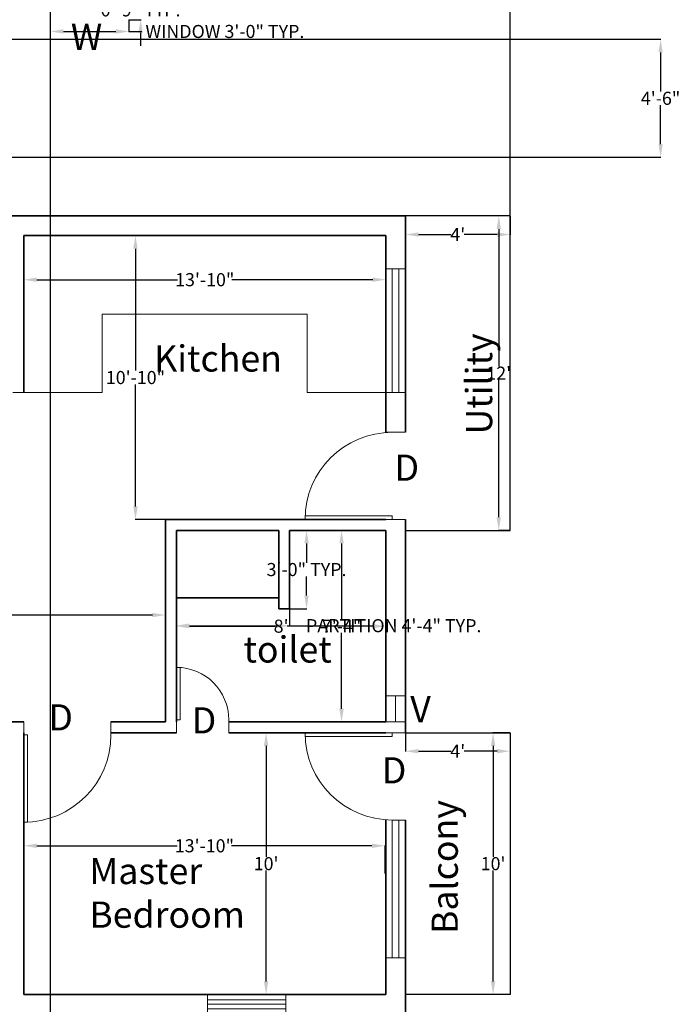
# Model space of a CAD drawing. Units: inches. Extents: x 1936 to 2761, y 1431 to 2889.
# Tile 4 of 6: x 2444 to 2747, y 1999 to 2451. Entities that reach past the tile are written whole.
import ezdxf

# ---------------------------------------------------------------- set-up
doc = ezdxf.new("R2010")
doc.units = ezdxf.units.IN
doc.header["$MEASUREMENT"] = 0
for name, color, linetype, lineweight in [('A-ANNO-DIMS', 172, 'Continuous', 13), ('A-ANNO-TEXT', 50, 'Continuous', 18), ('A-AREA-IDEN', 50, 'Continuous', 18), ('A-FLOR-EDGE', 4, 'Continuous', 25), ('A-FLOR-FIXT', 8, 'Continuous', 18), ('A-GLAZ', 3, 'Continuous', 18), ('A-WALL', 4, 'Continuous', 35), ('doors', 10, 'Continuous', 18)]:
    doc.layers.add(name, color=color, linetype=linetype, lineweight=lineweight)
doc.styles.get("Standard").update_dxf_attribs({"font": 'arial.ttf'})
doc.dimstyles.get("Standard").update_dxf_attribs({"dimtxt": 6, "dimasz": 6, "dimexe": 0.18, "dimexo": 0.0625, "dimgap": 0.09, "dimtad": 0, "dimtih": 1, "dimtoh": 1, "dimdec": 0, "dimzin": 0, "dimdsep": 46, "dimlunit": 3, "dimtxsty": 'Standard', "dimcen": 0.09, "dimadec": 0, "dimazin": 0, "dimtfac": 1, "dimtdec": 0, "dimtofl": 0, "dimtmove": 0, "dimatfit": 3, "dimfxl": 1, "dimtolj": 1, "dimtzin": 0, "dimarcsym": 0})

# ---------------------------------------------------------------- blocks, each defined once
blk = doc.blocks.new('*U2')
for p, q in [((0, 0), (0, 6)), ((40, 0), (40, 6))]:
    blk.add_line(p, q)
blk.add_lwpolyline([(0, 0), (0, -40), (1.75, -40), (1.75, 0)], close=True)
blk.add_arc((0, 0), 40, 270, 360)
blk = doc.blocks.new('*U3')
for p, q in [((0, 0), (0, -6)), ((24, 0), (24, -6))]:
    blk.add_line(p, q)
blk.add_lwpolyline([(0, 0), (0, 24), (1.75, 24), (1.75, 0)], close=True)
blk.add_arc((0, 0), 24, 0, 90)
blk = doc.blocks.new('*U5')
for p, q in [((0, 0), (0, -6)), ((40, 0), (40, -6))]:
    blk.add_line(p, q)
blk.add_lwpolyline([(0, 0), (0, 40), (1.75, 40), (1.75, 0)], close=True)
blk.add_arc((0, 0), 40, 0, 90)
blk = doc.blocks.new('*D39')
at = {"layer": 'A-ANNO-DIMS', "color": 0, "lineweight": -2, "transparency": 16777216}
for p, q in [((2321.01, 2177.61), (2321.01, 2177.73)), ((2327.01, 2177.55), (2403.56, 2177.55)), ((2505.01, 2177.55), (2428.45, 2177.55)), ((2511.01, 2177.61), (2511.01, 2177.73))]:
    blk.add_line(p, q, dxfattribs=at)
at = {"layer": 'A-ANNO-DIMS', "color": 0, "transparency": 16777216}
for points in [[(2327.01, 2178.55), (2327.01, 2176.55), (2321.01, 2177.55)], [(2505.01, 2178.55), (2505.01, 2176.55), (2511.01, 2177.55)]]:
    blk.add_solid(points, dxfattribs=at)
at = {"layer": 'Defpoints', "color": 0, "transparency": 16777216}
for p in [(2321.01, 2177.55), (2511.01, 2177.55), (2511.01, 2177.55)]:
    blk.add_point(p, dxfattribs=at)
at = {"layer": 'A-ANNO-DIMS', "color": 0, "transparency": 16777216, "insert": (2416.01, 2177.55), "char_height": 6, "attachment_point": 5}
blk.add_mtext('\\A1;15\'-10"', dxfattribs=at)
blk = doc.blocks.new('*D41')
at = {"layer": 'A-ANNO-DIMS', "color": 0, "lineweight": -2, "transparency": 16777216}
for p, q in [((2446.01, 2331.38), (2446.01, 2331.5)), ((2452.01, 2331.32), (2516.56, 2331.32)), ((2606.01, 2331.32), (2541.45, 2331.32)), ((2612.01, 2331.38), (2612.01, 2331.5))]:
    blk.add_line(p, q, dxfattribs=at)
at = {"layer": 'A-ANNO-DIMS', "color": 0, "transparency": 16777216}
for points in [[(2452.01, 2332.32), (2452.01, 2330.32), (2446.01, 2331.32)], [(2606.01, 2332.32), (2606.01, 2330.32), (2612.01, 2331.32)]]:
    blk.add_solid(points, dxfattribs=at)
at = {"layer": 'Defpoints', "color": 0, "transparency": 16777216}
for p in [(2446.01, 2331.32), (2612.01, 2331.32), (2612.01, 2331.32)]:
    blk.add_point(p, dxfattribs=at)
at = {"layer": 'A-ANNO-DIMS', "color": 0, "transparency": 16777216, "insert": (2529.01, 2331.32), "char_height": 6, "attachment_point": 5}
blk.add_mtext('\\A1;13\'-10"', dxfattribs=at)
blk = doc.blocks.new('*D42')
at = {"layer": 'A-ANNO-DIMS', "color": 0, "lineweight": -2, "transparency": 16777216}
for p, q in [((2557.38, 2351.55), (2497.06, 2351.55)), ((2497.24, 2345.55), (2497.24, 2289.61)), ((2497.24, 2227.36), (2497.24, 2283.3)), ((2561.44, 2221.36), (2497.06, 2221.36))]:
    blk.add_line(p, q, dxfattribs=at)
at = {"layer": 'A-ANNO-DIMS', "color": 0, "transparency": 16777216}
for points in [[(2496.24, 2345.55), (2498.24, 2345.55), (2497.24, 2351.55)], [(2496.24, 2227.36), (2498.24, 2227.36), (2497.24, 2221.36)]]:
    blk.add_solid(points, dxfattribs=at)
at = {"layer": 'Defpoints', "color": 0, "transparency": 16777216}
for p in [(2557.44, 2351.55), (2497.24, 2221.36), (2561.51, 2221.36)]:
    blk.add_point(p, dxfattribs=at)
at = {"layer": 'A-ANNO-DIMS', "color": 0, "transparency": 16777216, "insert": (2497.24, 2286.45), "char_height": 6, "attachment_point": 5}
blk.add_mtext('\\A1;10\'-10"', dxfattribs=at)
blk = doc.blocks.new('*D34')
at = {"layer": 'A-ANNO-DIMS', "color": 0, "lineweight": -2, "transparency": 16777216}
for p, q in [((2516.01, 2172.52), (2516.01, 2172.63)), ((2522.01, 2172.45), (2561.15, 2172.45)), ((2606.01, 2172.45), (2566.86, 2172.45)), ((2612.01, 2172.52), (2612.01, 2172.63))]:
    blk.add_line(p, q, dxfattribs=at)
at = {"layer": 'A-ANNO-DIMS', "color": 0, "transparency": 16777216}
for points in [[(2522.01, 2173.45), (2522.01, 2171.45), (2516.01, 2172.45)], [(2606.01, 2173.45), (2606.01, 2171.45), (2612.01, 2172.45)]]:
    blk.add_solid(points, dxfattribs=at)
at = {"layer": 'Defpoints', "color": 0, "transparency": 16777216}
for p in [(2516.01, 2172.45), (2612.01, 2172.45), (2612.01, 2172.45)]:
    blk.add_point(p, dxfattribs=at)
at = {"layer": 'A-ANNO-DIMS', "color": 0, "transparency": 16777216, "insert": (2564.01, 2172.45), "char_height": 6, "attachment_point": 5}
blk.add_mtext("\\A1;8'", dxfattribs=at)
blk = doc.blocks.new('*D35')
at = {"layer": 'A-ANNO-DIMS', "color": 0, "lineweight": -2, "transparency": 16777216}
for p, q in [((2590.02, 2216.36), (2591.92, 2216.36)), ((2591.74, 2210.36), (2591.74, 2175.54)), ((2591.74, 2134.55), (2591.74, 2169.36)), ((2590.02, 2128.55), (2591.92, 2128.55))]:
    blk.add_line(p, q, dxfattribs=at)
at = {"layer": 'A-ANNO-DIMS', "color": 0, "transparency": 16777216}
for points in [[(2590.74, 2210.36), (2592.74, 2210.36), (2591.74, 2216.36)], [(2590.74, 2134.55), (2592.74, 2134.55), (2591.74, 2128.55)]]:
    blk.add_solid(points, dxfattribs=at)
at = {"layer": 'Defpoints', "color": 0, "transparency": 16777216}
for p in [(2589.96, 2216.36), (2589.96, 2128.55), (2591.74, 2128.55)]:
    blk.add_point(p, dxfattribs=at)
at = {"layer": 'A-ANNO-DIMS', "color": 0, "transparency": 16777216, "insert": (2591.74, 2172.45), "char_height": 6, "attachment_point": 5}
blk.add_mtext('\\A1;7\'-4"', dxfattribs=at)
blk = doc.blocks.new('*D48')
at = {"layer": 'A-ANNO-DIMS', "color": 0, "lineweight": -2, "transparency": 16777216}
for p, q in [((2446.01, 2059.1), (2446.01, 2071.92)), ((2452.01, 2071.74), (2516.41, 2071.74)), ((2605.69, 2071.74), (2541.29, 2071.74)), ((2611.69, 2059.1), (2611.69, 2071.92))]:
    blk.add_line(p, q, dxfattribs=at)
at = {"layer": 'A-ANNO-DIMS', "color": 0, "transparency": 16777216}
for points in [[(2452.01, 2072.74), (2452.01, 2070.74), (2446.01, 2071.74)], [(2605.69, 2072.74), (2605.69, 2070.74), (2611.69, 2071.74)]]:
    blk.add_solid(points, dxfattribs=at)
at = {"layer": 'Defpoints', "color": 0, "transparency": 16777216}
for p in [(2446.01, 2071.74), (2446.01, 2059.04), (2611.69, 2059.04)]:
    blk.add_point(p, dxfattribs=at)
at = {"layer": 'A-ANNO-DIMS', "color": 0, "transparency": 16777216, "insert": (2528.85, 2071.74), "char_height": 6, "attachment_point": 5}
blk.add_mtext('\\A1;13\'-10"', dxfattribs=at)
blk = doc.blocks.new('*D49')
at = {"layer": 'A-ANNO-DIMS', "color": 0, "lineweight": -2, "transparency": 16777216}
for p, q in [((2552.34, 2123.55), (2557.32, 2123.55)), ((2557.14, 2117.55), (2557.14, 2066.7)), ((2557.14, 2009.55), (2557.14, 2060.4)), ((2552.34, 2003.55), (2557.32, 2003.55))]:
    blk.add_line(p, q, dxfattribs=at)
at = {"layer": 'A-ANNO-DIMS', "color": 0, "transparency": 16777216}
for points in [[(2556.14, 2117.55), (2558.14, 2117.55), (2557.14, 2123.55)], [(2556.14, 2009.55), (2558.14, 2009.55), (2557.14, 2003.55)]]:
    blk.add_solid(points, dxfattribs=at)
at = {"layer": 'Defpoints', "color": 0, "transparency": 16777216}
for p in [(2552.28, 2123.55), (2557.14, 2123.55), (2552.28, 2003.55)]:
    blk.add_point(p, dxfattribs=at)
at = {"layer": 'A-ANNO-DIMS', "color": 0, "transparency": 16777216, "insert": (2557.14, 2063.55), "char_height": 6, "attachment_point": 5}
blk.add_mtext("\\A1;10'", dxfattribs=at)
blk = doc.blocks.new('*D50')
at = {"layer": 'A-ANNO-DIMS', "color": 0, "lineweight": -2, "transparency": 16777216}
for p, q in [((2621.01, 2360.49), (2621.01, 2351.86)), ((2669.01, 2360.49), (2669.01, 2351.86)), ((2627.01, 2352.04), (2642.03, 2352.04)), ((2663.01, 2352.04), (2647.98, 2352.04))]:
    blk.add_line(p, q, dxfattribs=at)
at = {"layer": 'A-ANNO-DIMS', "color": 0, "transparency": 16777216}
for points in [[(2627.01, 2353.04), (2627.01, 2351.04), (2621.01, 2352.04)], [(2663.01, 2353.04), (2663.01, 2351.04), (2669.01, 2352.04)]]:
    blk.add_solid(points, dxfattribs=at)
at = {"layer": 'Defpoints', "color": 0, "transparency": 16777216}
for p in [(2621.01, 2360.55), (2669.01, 2360.55), (2669.01, 2352.04)]:
    blk.add_point(p, dxfattribs=at)
at = {"layer": 'A-ANNO-DIMS', "color": 0, "transparency": 16777216, "insert": (2645.01, 2352.04), "char_height": 6, "attachment_point": 5}
blk.add_mtext("\\A1;4'", dxfattribs=at)
blk = doc.blocks.new('*D51')
at = {"layer": 'A-ANNO-DIMS', "color": 0, "lineweight": -2, "transparency": 16777216}
for p, q in [((2668.94, 2360.55), (2663.63, 2360.55)), ((2663.81, 2354.55), (2663.81, 2291.56)), ((2663.81, 2222.36), (2663.81, 2285.35)), ((2668.94, 2216.36), (2663.63, 2216.36))]:
    blk.add_line(p, q, dxfattribs=at)
at = {"layer": 'A-ANNO-DIMS', "color": 0, "transparency": 16777216}
for points in [[(2662.81, 2354.55), (2664.81, 2354.55), (2663.81, 2360.55)], [(2662.81, 2222.36), (2664.81, 2222.36), (2663.81, 2216.36)]]:
    blk.add_solid(points, dxfattribs=at)
at = {"layer": 'Defpoints', "color": 0, "transparency": 16777216}
for p in [(2669.01, 2360.55), (2663.81, 2216.36), (2669.01, 2216.36)]:
    blk.add_point(p, dxfattribs=at)
at = {"layer": 'A-ANNO-DIMS', "color": 0, "transparency": 16777216, "insert": (2663.81, 2288.45), "char_height": 6, "attachment_point": 5}
blk.add_mtext("\\A1;12'", dxfattribs=at)
blk = doc.blocks.new('*D52')
at = {"layer": 'A-ANNO-DIMS', "color": 0, "lineweight": -2, "transparency": 16777216}
for p, q in [((2621.01, 2123.49), (2621.01, 2114.93)), ((2669.01, 2123.49), (2669.01, 2114.93)), ((2627.01, 2115.11), (2642.03, 2115.11)), ((2663.01, 2115.11), (2647.98, 2115.11))]:
    blk.add_line(p, q, dxfattribs=at)
at = {"layer": 'A-ANNO-DIMS', "color": 0, "transparency": 16777216}
for points in [[(2627.01, 2116.11), (2627.01, 2114.11), (2621.01, 2115.11)], [(2663.01, 2116.11), (2663.01, 2114.11), (2669.01, 2115.11)]]:
    blk.add_solid(points, dxfattribs=at)
at = {"layer": 'Defpoints', "color": 0, "transparency": 16777216}
for p in [(2621.01, 2123.55), (2669.01, 2123.55), (2669.01, 2115.11)]:
    blk.add_point(p, dxfattribs=at)
at = {"layer": 'A-ANNO-DIMS', "color": 0, "transparency": 16777216, "insert": (2645.01, 2115.11), "char_height": 6, "attachment_point": 5}
blk.add_mtext("\\A1;4'", dxfattribs=at)
blk = doc.blocks.new('*D53')
at = {"layer": 'A-ANNO-DIMS', "color": 0, "lineweight": -2, "transparency": 16777216}
for p, q in [((2668.94, 2123.55), (2661.03, 2123.55)), ((2661.21, 2117.55), (2661.21, 2066.7)), ((2661.21, 2009.55), (2661.21, 2060.4)), ((2668.94, 2003.55), (2661.03, 2003.55))]:
    blk.add_line(p, q, dxfattribs=at)
at = {"layer": 'A-ANNO-DIMS', "color": 0, "transparency": 16777216}
for points in [[(2660.21, 2117.55), (2662.21, 2117.55), (2661.21, 2123.55)], [(2660.21, 2009.55), (2662.21, 2009.55), (2661.21, 2003.55)]]:
    blk.add_solid(points, dxfattribs=at)
at = {"layer": 'Defpoints', "color": 0, "transparency": 16777216}
for p in [(2669.01, 2123.55), (2661.21, 2003.55), (2669.01, 2003.55)]:
    blk.add_point(p, dxfattribs=at)
at = {"layer": 'A-ANNO-DIMS', "color": 0, "transparency": 16777216, "insert": (2661.21, 2063.55), "char_height": 6, "attachment_point": 5}
blk.add_mtext("\\A1;10'", dxfattribs=at)
blk = doc.blocks.new('WIN-36')
for p, q in [((0, 9), (0, 0)), ((36, 6.5), (0, 6.5)), ((36, 9), (36, 0)), ((36, 4.5), (0, 4.5)), ((36, 2.5), (0, 2.5))]:
    blk.add_line(p, q)
blk = doc.blocks.new('VENT-12')
for p, q in [((0, 0), (0, 9)), ((12, 0), (12, 9)), ((0, 4.5), (12, 4.5))]:
    blk.add_line(p, q)
blk = doc.blocks.new('WIN-KITCHEN')
for p, q in [((0, 56.83), (9, 56.83)), ((3, 56.83), (3, 0)), ((6, 56.83), (6, 0)), ((0, 0), (9, 0))]:
    blk.add_line(p, q)
blk = doc.blocks.new('WIN-BALCONY')
for p, q in [((3, 63.14), (3, 0)), ((6, 63.14), (6, 0)), ((0, 0), (9, 0))]:
    blk.add_line(p, q)
blk = doc.blocks.new('COUNTER-KITCHEN-U')
for p, q in [((41, 36), (41, 0)), ((41, 36), (135, 36)), ((135, 36), (135, 0)), ((0, 0), (41, 0)), ((135, 0), (171, 0))]:
    blk.add_line(p, q)
blk = doc.blocks.new('BATH-PARTITION')
for p, q in [((0, 35.9), (46.9, 35.9)), ((0, 5), (0, 35.9)), ((46.9, 35.9), (46.9, 0)), ((51.9, 35.9), (51.9, 0)), ((46.9, 5), (0, 5)), ((51.9, 0), (46.9, 0))]:
    blk.add_line(p, q)
blk = doc.blocks.new('*D87')
at = {"layer": 'A-ANNO-DIMS', "color": 0, "lineweight": -2, "transparency": 16777216}
for p, q in [((2458.21, 2450.49), (2458.21, 2444.97)), ((2494.21, 2450.49), (2494.21, 2444.97)), ((2464.21, 2445.15), (2488.21, 2445.15)), ((2494.21, 2445.15), (2500.21, 2445.15))]:
    blk.add_line(p, q, dxfattribs=at)
at = {"layer": 'A-ANNO-DIMS', "color": 0, "transparency": 16777216}
for points in [[(2464.21, 2446.15), (2464.21, 2444.15), (2458.21, 2445.15)], [(2488.21, 2446.15), (2488.21, 2444.15), (2494.21, 2445.15)]]:
    blk.add_solid(points, dxfattribs=at)
at = {"layer": 'Defpoints', "color": 0, "transparency": 16777216}
for p in [(2458.21, 2450.55), (2494.21, 2450.55), (2494.21, 2445.15)]:
    blk.add_point(p, dxfattribs=at)
at = {"layer": 'A-ANNO-DIMS', "color": 0, "transparency": 16777216, "insert": (2538.26, 2445.15), "char_height": 6, "attachment_point": 5}
blk.add_mtext('\\A1;WINDOW 3\'-0" TYP.', dxfattribs=at)
blk = doc.blocks.new('*D88')
at = {"layer": 'A-ANNO-DIMS', "color": 0, "lineweight": -2, "transparency": 16777216}
for p, q in [((2499.61, 2465.55), (2499.61, 2471.55)), ((2494.27, 2459.55), (2499.79, 2459.55)), ((2494.27, 2450.55), (2499.79, 2450.55)), ((2499.61, 2444.55), (2499.61, 2438.55))]:
    blk.add_line(p, q, dxfattribs=at)
at = {"layer": 'A-ANNO-DIMS', "color": 0, "transparency": 16777216}
for points in [[(2498.61, 2465.55), (2500.61, 2465.55), (2499.61, 2459.55)], [(2498.61, 2444.55), (2500.61, 2444.55), (2499.61, 2450.55)]]:
    blk.add_solid(points, dxfattribs=at)
at = {"layer": 'Defpoints', "color": 0, "transparency": 16777216}
for p in [(2494.21, 2459.55), (2499.61, 2459.55), (2494.21, 2450.55)]:
    blk.add_point(p, dxfattribs=at)
at = {"layer": 'A-ANNO-DIMS', "color": 0, "transparency": 16777216, "insert": (2499.61, 2455.05), "char_height": 6, "attachment_point": 5}
blk.add_mtext('\\A1;0\'-9" TYP.', dxfattribs=at)
blk = doc.blocks.new('*D95')
at = {"layer": 'A-ANNO-DIMS', "color": 0, "lineweight": -2, "transparency": 16777216}
for p, q in [((2516.01, 2180.39), (2516.01, 2172.49)), ((2567.9, 2180.39), (2567.9, 2172.49)), ((2522.01, 2172.67), (2561.9, 2172.67)), ((2567.9, 2172.67), (2573.9, 2172.67))]:
    blk.add_line(p, q, dxfattribs=at)
at = {"layer": 'A-ANNO-DIMS', "color": 0, "transparency": 16777216}
for points in [[(2522.01, 2173.67), (2522.01, 2171.67), (2516.01, 2172.67)], [(2561.9, 2173.67), (2561.9, 2171.67), (2567.9, 2172.67)]]:
    blk.add_solid(points, dxfattribs=at)
at = {"layer": 'Defpoints', "color": 0, "transparency": 16777216}
for p in [(2516.01, 2180.46), (2567.9, 2180.46), (2567.9, 2172.67)]:
    blk.add_point(p, dxfattribs=at)
at = {"layer": 'A-ANNO-DIMS', "color": 0, "transparency": 16777216, "insert": (2615.65, 2172.67), "char_height": 6, "attachment_point": 5}
blk.add_mtext('\\A1;PARTITION 4\'-4" TYP.', dxfattribs=at)
blk = doc.blocks.new('*D96')
at = {"layer": 'A-ANNO-DIMS', "color": 0, "lineweight": -2, "transparency": 16777216}
for p, q in [((2567.97, 2216.36), (2575.87, 2216.36)), ((2575.69, 2210.36), (2575.69, 2201.56)), ((2575.69, 2186.46), (2575.69, 2195.25)), ((2567.97, 2180.46), (2575.87, 2180.46))]:
    blk.add_line(p, q, dxfattribs=at)
at = {"layer": 'A-ANNO-DIMS', "color": 0, "transparency": 16777216}
for points in [[(2574.69, 2210.36), (2576.69, 2210.36), (2575.69, 2216.36)], [(2574.69, 2186.46), (2576.69, 2186.46), (2575.69, 2180.46)]]:
    blk.add_solid(points, dxfattribs=at)
at = {"layer": 'Defpoints', "color": 0, "transparency": 16777216}
for p in [(2567.9, 2216.36), (2575.69, 2216.36), (2567.9, 2180.46)]:
    blk.add_point(p, dxfattribs=at)
at = {"layer": 'A-ANNO-DIMS', "color": 0, "transparency": 16777216, "insert": (2575.69, 2198.41), "char_height": 6, "attachment_point": 5}
blk.add_mtext('\\A1;3\'-0" TYP.', dxfattribs=at)
blk = doc.blocks.new('*D99')
at = {"layer": 'A-ANNO-DIMS', "color": 0, "lineweight": -2, "transparency": 16777216}
for p, q in [((2021.01, 2816.61), (2021.01, 2885.73)), ((2027.01, 2885.55), (2334.61, 2885.55)), ((2663.01, 2885.55), (2355.4, 2885.55)), ((2669.01, 2360.61), (2669.01, 2885.73))]:
    blk.add_line(p, q, dxfattribs=at)
at = {"layer": 'A-ANNO-DIMS', "color": 0, "transparency": 16777216}
for points in [[(2027.01, 2886.55), (2027.01, 2884.55), (2021.01, 2885.55)], [(2663.01, 2886.55), (2663.01, 2884.55), (2669.01, 2885.55)]]:
    blk.add_solid(points, dxfattribs=at)
at = {"layer": 'Defpoints', "color": 0, "transparency": 16777216}
for p in [(2669.01, 2885.55), (2021.01, 2816.55), (2669.01, 2360.55)]:
    blk.add_point(p, dxfattribs=at)
at = {"layer": 'A-ANNO-DIMS', "color": 0, "transparency": 16777216, "insert": (2345.01, 2885.55), "char_height": 6, "attachment_point": 5}
blk.add_mtext('\\A1;54\'-0"', dxfattribs=at)
blk = doc.blocks.new('*D108')
at = {"layer": 'A-ANNO-DIMS', "color": 0, "lineweight": -2, "transparency": 16777216}
for p, q in [((2141.07, 2441.55), (2738.19, 2441.55)), ((2738.01, 2435.55), (2738.01, 2417.65)), ((2738.01, 2393.45), (2738.01, 2411.34)), ((2141.07, 2387.45), (2738.19, 2387.45))]:
    blk.add_line(p, q, dxfattribs=at)
at = {"layer": 'A-ANNO-DIMS', "color": 0, "transparency": 16777216}
for points in [[(2737.01, 2435.55), (2739.01, 2435.55), (2738.01, 2441.55)], [(2737.01, 2393.45), (2739.01, 2393.45), (2738.01, 2387.45)]]:
    blk.add_solid(points, dxfattribs=at)
at = {"layer": 'Defpoints', "color": 0, "transparency": 16777216}
for p in [(2141.01, 2441.55), (2738.01, 2441.55), (2141.01, 2387.45)]:
    blk.add_point(p, dxfattribs=at)
at = {"layer": 'A-ANNO-DIMS', "color": 0, "transparency": 16777216, "insert": (2738.01, 2414.5), "char_height": 6, "attachment_point": 5}
blk.add_mtext('\\A1;4\'-6"', dxfattribs=at)
blk = doc.blocks.new('*D112')
at = {"layer": 'A-ANNO-DIMS', "color": 0, "lineweight": -2, "transparency": 16777216}
for p, q in [((2374.01, 2459.49), (2374.01, 1439.37)), ((2458.21, 2459.49), (2458.21, 1439.37)), ((2380.01, 1439.55), (2408.07, 1439.55)), ((2452.21, 1439.55), (2424.15, 1439.55))]:
    blk.add_line(p, q, dxfattribs=at)
at = {"layer": 'A-ANNO-DIMS', "color": 0, "transparency": 16777216}
for points in [[(2380.01, 1440.55), (2380.01, 1438.55), (2374.01, 1439.55)], [(2452.21, 1440.55), (2452.21, 1438.55), (2458.21, 1439.55)]]:
    blk.add_solid(points, dxfattribs=at)
at = {"layer": 'Defpoints', "color": 0, "transparency": 16777216}
for p in [(2374.01, 2459.55), (2458.21, 2459.55), (2458.21, 1439.55)]:
    blk.add_point(p, dxfattribs=at)
at = {"layer": 'A-ANNO-DIMS', "color": 0, "transparency": 16777216, "insert": (2416.11, 1439.55), "char_height": 6, "attachment_point": 5}
blk.add_mtext('\\A1;7\'-0"', dxfattribs=at)

msp = doc.modelspace()

# ---------------------------------------------------------------- linework, layer by layer
at = {"layer": 'A-FLOR-EDGE'}
for p, q in [((2669.01, 2360.55), (2621.01, 2360.55)), ((2669.01, 2216.36), (2669.01, 2360.55)), ((2621.01, 2216.36), (2669.01, 2216.36)), ((2621.01, 2123.55), (2669.01, 2123.55)), ((2669.01, 2123.55), (2669.01, 2003.55)), ((2669.01, 2003.55), (2621.01, 2003.55))]:
    msp.add_line(p, q, dxfattribs=at)
at = {"layer": 'A-WALL'}
for p, q in [((2141.01, 2360.55), (2621.01, 2360.55)), ((2621.01, 2360.55), (2621.01, 2261.36)), ((2446.01, 2351.55), (2446.01, 2279.55)), ((2446.01, 2351.55), (2612.01, 2351.55)), ((2612.01, 2351.55), (2612.01, 2261.36)), ((2511.01, 2221.36), (2511.01, 2128.55)), ((2511.01, 2221.36), (2612.01, 2221.36)), ((2621.01, 2221.36), (2621.01, 2123.55)), ((2516.01, 2216.36), (2516.01, 2128.55)), ((2516.01, 2216.36), (2562.9, 2216.36)), ((2567.9, 2216.36), (2612.01, 2216.36)), ((2612.01, 2216.36), (2612.01, 2128.55)), ((2446.01, 2128.55), (2361.01, 2128.55)), ((2511.01, 2128.55), (2486.01, 2128.55)), ((2612.01, 2128.55), (2540.01, 2128.55)), ((2446.01, 2123.55), (2446.01, 2003.55)), ((2516.01, 2123.55), (2486.01, 2123.55)), ((2612.01, 2123.55), (2540.01, 2123.55)), ((2612.01, 2083.66), (2612.01, 2003.55)), ((2621.01, 2083.55), (2621.01, 1994.55)), ((2612.01, 2003.55), (2446.01, 2003.55))]:
    msp.add_line(p, q, dxfattribs=at)
at = {"layer": 'doors'}
for p, q in [((2612.01, 2261.36), (2621.01, 2261.36)), ((2612.01, 2221.36), (2621.01, 2221.36)), ((2446.01, 2128.55), (2446.01, 2123.55)), ((2486.01, 2128.55), (2486.01, 2123.55)), ((2516.01, 2128.55), (2516.01, 2123.55)), ((2540.01, 2128.55), (2540.01, 2123.55)), ((2612.01, 2123.55), (2621.01, 2123.55))]:
    msp.add_line(p, q, dxfattribs=at)

# ---------------------------------------------------------------- block references
at = {"layer": 'A-FLOR-FIXT'}
msp.add_blockref('COUNTER-KITCHEN-U', (2441.01, 2279.55), dxfattribs=at)
at = {"layer": 'A-GLAZ'}
for name, p in [('WIN-KITCHEN', (2612.01, 2279.55)), ('WIN-BALCONY', (2612.01, 2020.41)), ('WIN-36', (2530.21, 1994.55))]:
    msp.add_blockref(name, p, dxfattribs=at)
at = {"layer": 'A-GLAZ', "rotation": 270.0000000000007}
msp.add_blockref('VENT-12', (2612.01, 2140.55), dxfattribs=at)
at = {"layer": 'A-WALL'}
msp.add_blockref('BATH-PARTITION', (2516.01, 2180.46), dxfattribs=at)
at = {"layer": 'doors', "rotation": 90}
msp.add_blockref('*U5', (2615.01, 2221.36), dxfattribs=at)
at = {"layer": 'doors'}
for name, p in [('*U3', (2516.01, 2129.55)), ('*U2', (2446.01, 2122.55))]:
    msp.add_blockref(name, p, dxfattribs=at)
at = {"layer": 'doors', "xscale": -1, "rotation": 90}
msp.add_blockref('*U5', (2615.01, 2123.55), dxfattribs=at)

# ---------------------------------------------------------------- texts
at = {"layer": 'A-ANNO-TEXT', "char_height": 12, "attachment_point": 1}
for s, width, heights, insert in [('W', 7.8209, [0.2], (2467.63, 2448.68)), ('D', 28.2371, [0.2], (2616.03, 2251.11)), ('V', 13.1151, [0], (2623.24, 2140.37)), ('D', 28.2371, [0.2], (2457.33, 2136.61)), ('D', 28.2371, [0.2], (2523.04, 2135.24)), ('D', 28.2371, [0.2], (2610.2, 2112.35))]:
    msp.add_mtext_dynamic_manual_height_columns(s, width=width, gutter_width=1, heights=heights, dxfattribs=dict(at, insert=insert))
at = {"layer": 'A-AREA-IDEN', "char_height": 12, "attachment_point": 1, "rotation": 90}
for s, insert in [('Utility', (2648.79, 2260.35)), ('Balcony', (2633.04, 2031.28))]:
    msp.add_mtext_dynamic_manual_height_columns(s, width=55.7076, gutter_width=1, heights=[0], dxfattribs=dict(at, insert=insert))
at = {"layer": 'A-AREA-IDEN', "char_height": 12, "attachment_point": 1}
for s, insert in [('Kitchen', (2505.82, 2301.2)), ('toilet', (2546.76, 2167.77)), ('Master Bedroom', (2476.08, 2066.17))]:
    msp.add_mtext_dynamic_manual_height_columns(s, width=55.7076, gutter_width=1, heights=[0], dxfattribs=dict(at, insert=insert))

# ---------------------------------------------------------------- dimensions: what is measured, and where the dimension line sits
at = {"layer": 'A-ANNO-DIMS'}
for base, p1, p2, override, picture, middle in [((2669.01, 2885.55), (2021.01, 2816.55), (2669.01, 2360.55), {"dimdec": 1, "dimlfac": 1, "dimrnd": 0, "dimzin": 1, "dimdsep": 46, "dimlunit": 4, "dimfrac": 2}, '*D99', (2345.01, 2885.55)), ((2458.21, 1439.55), (2374.01, 2459.55), (2458.21, 2459.55), {"dimdec": 1, "dimlfac": 1, "dimrnd": 0, "dimzin": 1, "dimdsep": 46, "dimlunit": 4, "dimfrac": 2}, '*D112', (2416.11, 1439.55)), ((2669.01, 2352.04), (2621.01, 2360.55), (2669.01, 2360.55), {"dimclrd": 0, "dimclre": 0, "dimclrt": 0}, '*D50', (2645.01, 2352.04)), ((2612.01, 2331.32), (2446.01, 2331.32), (2612.01, 2331.32), {"dimclrd": 0, "dimclre": 0, "dimclrt": 0}, '*D41', (2529.01, 2331.32)), ((2511.01, 2177.55), (2321.01, 2177.55), (2511.01, 2177.55), {"dimclrd": 0, "dimclre": 0, "dimclrt": 0}, '*D39', (2416.01, 2177.55)), ((2612.01, 2172.45), (2516.01, 2172.45), (2612.01, 2172.45), {"dimclrd": 0, "dimclre": 0, "dimclrt": 0}, '*D34', (2564.01, 2172.45)), ((2669.01, 2115.11), (2621.01, 2123.55), (2669.01, 2123.55), {"dimclrd": 0, "dimclre": 0, "dimclrt": 0}, '*D52', (2645.01, 2115.11)), ((2446.01, 2071.74), (2611.69, 2059.04), (2446.01, 2059.04), {"dimclrd": 0, "dimclre": 0, "dimclrt": 0}, '*D48', (2528.85, 2071.74))]:
    dim = msp.add_linear_dim(base=base, p1=p1, p2=p2, dimstyle='Standard', override=override, dxfattribs=at)
    dim.commit()
    dim.dimension.update_dxf_attribs({"geometry": picture, "text_midpoint": middle})
for base, p1, p2, picture, middle in [((2499.61, 2459.55), (2494.21, 2450.55), (2494.21, 2459.55), '*D88', (2499.61, 2455.05)), ((2575.69, 2216.36), (2567.9, 2180.46), (2567.9, 2216.36), '*D96', (2575.69, 2198.41))]:
    dim = msp.add_linear_dim(base=base, p1=p1, p2=p2, angle=90, text='<> TYP.', dimstyle='Standard', override={"dimdec": 1, "dimlfac": 1, "dimrnd": 0, "dimzin": 1, "dimdsep": 46, "dimlunit": 4, "dimfrac": 2}, dxfattribs=at)
    dim.commit()
    dim.dimension.update_dxf_attribs({"geometry": picture, "text_midpoint": middle})
for base, p1, p2, text, picture, middle in [((2494.21, 2445.15), (2458.21, 2450.55), (2494.21, 2450.55), 'WINDOW <> TYP.', '*D87', (2538.26, 2445.15)), ((2567.9, 2172.67), (2516.01, 2180.46), (2567.9, 2180.46), 'PARTITION <> TYP.', '*D95', (2615.65, 2172.67))]:
    dim = msp.add_linear_dim(base=base, p1=p1, p2=p2, text=text, dimstyle='Standard', override={"dimdec": 1, "dimlfac": 1, "dimrnd": 0, "dimzin": 1, "dimdsep": 46, "dimlunit": 4, "dimfrac": 2}, dxfattribs=at)
    dim.commit()
    dim.dimension.update_dxf_attribs({"geometry": picture, "text_midpoint": middle})
for base, p1, p2, override, picture, middle in [((2738.01, 2441.55), (2141.01, 2387.45), (2141.01, 2441.55), {"dimdec": 1, "dimlfac": 1, "dimrnd": 0, "dimzin": 1, "dimdsep": 46, "dimlunit": 4, "dimfrac": 2}, '*D108', (2738.01, 2414.5)), ((2663.81, 2216.36), (2669.01, 2360.55), (2669.01, 2216.36), {"dimclrd": 0, "dimclre": 0, "dimclrt": 0}, '*D51', (2663.81, 2288.45)), ((2497.24, 2221.36), (2557.44, 2351.55), (2561.51, 2221.36), {"dimclrd": 0, "dimclre": 0, "dimclrt": 0}, '*D42', (2497.24, 2286.45)), ((2591.74, 2128.55), (2589.96, 2216.36), (2589.96, 2128.55), {"dimclrd": 0, "dimclre": 0, "dimclrt": 0}, '*D35', (2591.74, 2172.45)), ((2557.14, 2123.55), (2552.28, 2003.55), (2552.28, 2123.55), {"dimclrd": 0, "dimclre": 0, "dimclrt": 0}, '*D49', (2557.14, 2063.55)), ((2661.21, 2003.55), (2669.01, 2123.55), (2669.01, 2003.55), {"dimclrd": 0, "dimclre": 0, "dimclrt": 0}, '*D53', (2661.21, 2063.55))]:
    dim = msp.add_linear_dim(base=base, p1=p1, p2=p2, angle=90, dimstyle='Standard', override=override, dxfattribs=at)
    dim.commit()
    dim.dimension.update_dxf_attribs({"geometry": picture, "text_midpoint": middle})

doc.saveas('drawing.dxf')
